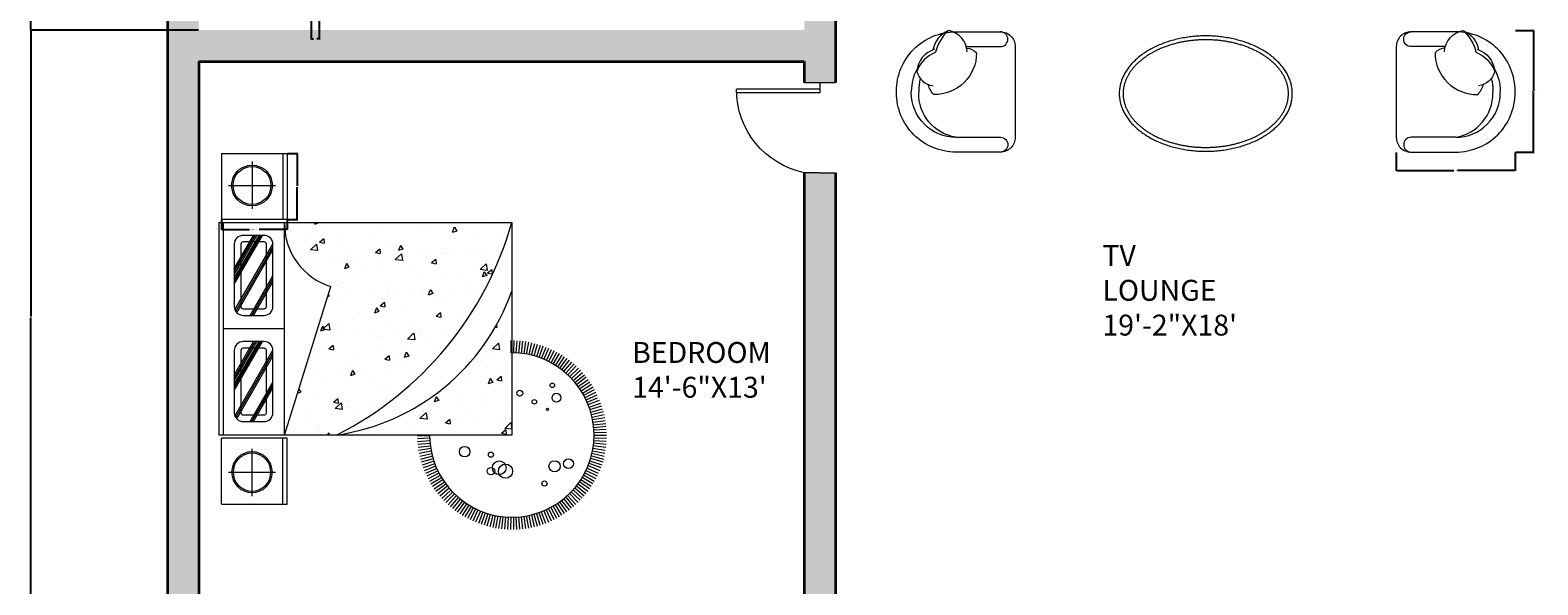
# Model space of a CAD drawing. Units: inches. Extents: x -9 to 646, y -802 to 47.
# Tile 14 of 17: x -9 to 424, y -412 to -253. Entities that reach past the tile are written whole.
import ezdxf

# ---------------------------------------------------------------- set-up
doc = ezdxf.new("R2010")
doc.units = ezdxf.units.IN
doc.header["$MEASUREMENT"] = 0
for name, color, linetype, lineweight in [('A-ANNO-DIMS', 2, 'Continuous', 18), ('A-AREA-IDEN', 7, 'Continuous', 18), ('A-DOOR', 4, 'Continuous', 18), ('A-FURN', 8, 'Continuous', 15), ('A-FURN-PATT', 252, 'Continuous', 9), ('A-WALL', 7, 'Continuous', 35), ('A-WALL-PATT', 5, 'Continuous', 9)]:
    doc.layers.add(name, color=color, linetype=linetype, lineweight=lineweight)
doc.styles.get("Standard").update_dxf_attribs({"font": 'arial.ttf'})
doc.dimstyles.get("Standard").update_dxf_attribs({"dimtxt": 0.18, "dimasz": 0.18, "dimexe": 0.18, "dimexo": 0.0625, "dimgap": 0.09, "dimtad": 0, "dimtih": 1, "dimtoh": 1, "dimdec": 0, "dimzin": 0, "dimdsep": 46, "dimlunit": 3, "dimtxsty": 'Standard', "dimcen": 0.09, "dimadec": 0, "dimazin": 0, "dimtfac": 1, "dimtdec": 0, "dimtofl": 0, "dimtmove": 0, "dimatfit": 3, "dimfxl": 1, "dimtolj": 1, "dimtzin": 0, "dimarcsym": 0})

# ---------------------------------------------------------------- blocks, each defined once
blk = doc.blocks.new('LOUNGE-ARMCHAIR')
for points in [[(13.85, 28.82, -0.356772), (19.23, 34.93, -0.249542), (23.66, 29.39, 9.61688)], [(19.23, 34.93, -0.14773), (22.9, 28.69, -0.213343), (28.28, 23.19, -0.178662)], [(14.08, 30.31), (4.27, 30.31, -0.414214), (2.13, 32.45), (2.13, 32.45, -0.414214), (4.27, 34.58)], [(13.98, 29.89, 0.165541), (11.16, 28.57, 0.425989), (23.39, 16.58, 0.121523), (25.07, 19.43, -7.115464)], [(23.19, 29.56, -0.306663), (28.28, 23.19, -0.30633), (23.63, 19.03, 0.872847)], [(28.19, 23.86, -0.130591), (29.88, 17.51), (29.88, 17.29)], [(27.29, 21.15, -0.072384), (27.75, 17.51), (27.75, 17.29)], [(17.07, 4.27, 0.372719), (27.75, 17.08), (27.75, 17.29)], [(17.07, 4.27, 0.414214), (29.88, 17.08), (29.88, 17.29)], [(17.07, 4.27), (4.27, 4.27, 0.414214), (2.13, 2.14), (2.13, 2.14, 0.414214), (4.27, 0)]]:
    blk.add_lwpolyline(points, format="xyb")
at = {"ltscale": 0.03}
blk.add_lwpolyline([(0, 17.29), (0, 4.27, 0.414214), (4.27, 0), (17.07, 0, 0.414214), (34.15, 17.08), (34.15, 17.29), (34.15, 17.51, 0.414214), (17.07, 34.58), (4.27, 34.58, 0.414214), (0, 30.31), (0, 17.29)], format="xyb", dxfattribs=at)
blk = doc.blocks.new('NIGHTSTAND-19')
for p, q in [((0, 18.94), (18.94, 18.94)), ((0, 18.94), (0, 0)), ((17.61, 18.94), (17.61, 0)), ((18.94, 18.94), (18.94, 0)), ((8.8, 16.66), (8.8, 3.04)), ((2.08, 9.77), (15.53, 9.77)), ((18.94, 0), (0, 0))]:
    blk.add_line(p, q)
for radius in [5.86, 5.44]:
    blk.add_circle((8.8, 9.77), radius)
blk = doc.blocks.new('DOOR-LEAF-24-WALL9')
for p, q in [((0, 0), (0, 24)), ((1, 0), (1, 24)), ((0, 0), (1, 0))]:
    blk.add_line(p, q)
blk.add_arc((0, -0.52), 24.52, 11.8123, 90)
blk = doc.blocks.new('*D18')
at = {"layer": 'A-ANNO-DIMS', "color": 0, "lineweight": -2, "transparency": 16777216}
for p, q in [((71.7, -249.89), (71.7, -255.77)), ((73.94, -249.89), (73.94, -255.77)), ((71.88, -255.59), (72.36, -255.59)), ((73.76, -255.59), (73.28, -255.59))]:
    blk.add_line(p, q, dxfattribs=at)
at = {"layer": 'A-ANNO-DIMS', "color": 0, "transparency": 16777216}
for points in [[(71.88, -255.56), (71.88, -255.62), (71.7, -255.59)], [(73.76, -255.56), (73.76, -255.62), (73.94, -255.59)]]:
    blk.add_solid(points, dxfattribs=at)
at = {"layer": 'Defpoints', "color": 0, "transparency": 16777216}
for p in [(71.7, -249.82), (73.94, -249.82), (73.94, -255.59)]:
    blk.add_point(p, dxfattribs=at)
at = {"layer": 'A-ANNO-DIMS', "color": 0, "transparency": 16777216, "insert": (72.82, -255.59), "char_height": 0.18, "attachment_point": 5}
blk.add_mtext('\\A1;2 TYP.', dxfattribs=at)
blk = doc.blocks.new('*D35')
at = {"layer": 'A-ANNO-DIMS', "color": 0, "lineweight": -2, "transparency": 16777216}
for p, q in [((417.7, -253.19), (423.06, -253.19)), ((422.88, -253.37), (422.88, -270.47)), ((422.88, -287.94), (422.88, -270.84)), ((417.7, -288.12), (423.06, -288.12))]:
    blk.add_line(p, q, dxfattribs=at)
at = {"layer": 'A-ANNO-DIMS', "color": 0, "transparency": 16777216}
for points in [[(422.85, -253.37), (422.91, -253.37), (422.88, -253.19)], [(422.85, -287.94), (422.91, -287.94), (422.88, -288.12)]]:
    blk.add_solid(points, dxfattribs=at)
at = {"layer": 'Defpoints', "color": 0, "transparency": 16777216}
for p in [(417.64, -253.19), (422.88, -253.19), (417.64, -288.12)]:
    blk.add_point(p, dxfattribs=at)
at = {"layer": 'A-ANNO-DIMS', "color": 0, "transparency": 16777216, "insert": (422.88, -270.65), "char_height": 0.18, "attachment_point": 5}
blk.add_mtext('\\A1;ARMCHAIR 35 TYP.', dxfattribs=at)
blk = doc.blocks.new('*D36')
at = {"layer": 'A-ANNO-DIMS', "color": 0, "lineweight": -2, "transparency": 16777216}
for p, q in [((383.49, -288.18), (383.49, -293.54)), ((417.64, -288.18), (417.64, -293.54)), ((383.67, -293.36), (400.04, -293.36)), ((417.46, -293.36), (401.09, -293.36))]:
    blk.add_line(p, q, dxfattribs=at)
at = {"layer": 'A-ANNO-DIMS', "color": 0, "transparency": 16777216}
for points in [[(383.67, -293.33), (383.67, -293.39), (383.49, -293.36)], [(417.46, -293.33), (417.46, -293.39), (417.64, -293.36)]]:
    blk.add_solid(points, dxfattribs=at)
at = {"layer": 'Defpoints', "color": 0, "transparency": 16777216}
for p in [(383.49, -288.12), (417.64, -288.12), (417.64, -293.36)]:
    blk.add_point(p, dxfattribs=at)
at = {"layer": 'A-ANNO-DIMS', "color": 0, "transparency": 16777216, "insert": (400.56, -293.36), "char_height": 0.18, "attachment_point": 5}
blk.add_mtext('\\A1;34 TYP.', dxfattribs=at)
blk = doc.blocks.new('*D41')
at = {"layer": 'A-ANNO-DIMS', "color": 0, "lineweight": -2, "transparency": 16777216}
for p, q in [((45.87, -307.54), (45.87, -310.49)), ((64.81, -307.54), (64.81, -310.49)), ((46.05, -310.31), (53.96, -310.31)), ((64.63, -310.31), (56.71, -310.31))]:
    blk.add_line(p, q, dxfattribs=at)
at = {"layer": 'A-ANNO-DIMS', "color": 0, "transparency": 16777216}
for points in [[(46.05, -310.28), (46.05, -310.34), (45.87, -310.31)], [(64.63, -310.28), (64.63, -310.34), (64.81, -310.31)]]:
    blk.add_solid(points, dxfattribs=at)
at = {"layer": 'Defpoints', "color": 0, "transparency": 16777216}
for p in [(45.87, -307.47), (64.81, -307.47), (64.81, -310.31)]:
    blk.add_point(p, dxfattribs=at)
at = {"layer": 'A-ANNO-DIMS', "color": 0, "transparency": 16777216, "insert": (55.34, -310.31), "char_height": 0.18, "attachment_point": 5}
blk.add_mtext('\\A1;NIGHTSTAND 19 TYP.', dxfattribs=at)
blk = doc.blocks.new('*D42')
at = {"layer": 'A-ANNO-DIMS', "color": 0, "lineweight": -2, "transparency": 16777216}
for p, q in [((64.87, -288.53), (67.83, -288.53)), ((67.65, -288.71), (67.65, -297.82)), ((67.65, -307.29), (67.65, -298.18)), ((64.87, -307.47), (67.83, -307.47))]:
    blk.add_line(p, q, dxfattribs=at)
at = {"layer": 'A-ANNO-DIMS', "color": 0, "transparency": 16777216}
for points in [[(67.62, -288.71), (67.68, -288.71), (67.65, -288.53)], [(67.62, -307.29), (67.68, -307.29), (67.65, -307.47)]]:
    blk.add_solid(points, dxfattribs=at)
at = {"layer": 'Defpoints', "color": 0, "transparency": 16777216}
for p in [(64.81, -288.53), (67.65, -288.53), (64.81, -307.47)]:
    blk.add_point(p, dxfattribs=at)
at = {"layer": 'A-ANNO-DIMS', "color": 0, "transparency": 16777216, "insert": (67.65, -298), "char_height": 0.18, "attachment_point": 5}
blk.add_mtext('\\A1;19 TYP.', dxfattribs=at)
blk = doc.blocks.new('*D54')
at = {"layer": 'A-ANNO-DIMS', "color": 0, "lineweight": -2, "transparency": 16777216}
for p, q in [((30.31, 7.93), (-9.06, 7.93)), ((-8.88, 7.75), (-8.88, -122.39)), ((-8.88, -252.89), (-8.88, -122.75)), ((39.31, -253.07), (-9.06, -253.07))]:
    blk.add_line(p, q, dxfattribs=at)
at = {"layer": 'A-ANNO-DIMS', "color": 0, "transparency": 16777216}
for points in [[(-8.91, 7.75), (-8.85, 7.75), (-8.88, 7.93)], [(-8.91, -252.89), (-8.85, -252.89), (-8.88, -253.07)]]:
    blk.add_solid(points, dxfattribs=at)
at = {"layer": 'Defpoints', "color": 0, "transparency": 16777216}
for p in [(30.37, 7.93), (-8.88, -253.07), (39.37, -253.07)]:
    blk.add_point(p, dxfattribs=at)
at = {"layer": 'A-ANNO-DIMS', "color": 0, "transparency": 16777216, "insert": (-8.88, -122.57), "char_height": 0.18, "attachment_point": 5}
blk.add_mtext('\\A1;261', dxfattribs=at)
blk = doc.blocks.new('*D55')
at = {"layer": 'A-ANNO-DIMS', "color": 0, "lineweight": -2, "transparency": 16777216}
for p, q in [((39.31, -253.07), (-9.06, -253.07)), ((-8.88, -253.25), (-8.88, -335.39)), ((-8.88, -417.89), (-8.88, -335.75)), ((39.31, -418.07), (-9.06, -418.07))]:
    blk.add_line(p, q, dxfattribs=at)
at = {"layer": 'A-ANNO-DIMS', "color": 0, "transparency": 16777216}
for points in [[(-8.91, -253.25), (-8.85, -253.25), (-8.88, -253.07)], [(-8.91, -417.89), (-8.85, -417.89), (-8.88, -418.07)]]:
    blk.add_solid(points, dxfattribs=at)
at = {"layer": 'Defpoints', "color": 0, "transparency": 16777216}
for p in [(39.37, -253.07), (-8.88, -418.07), (39.37, -418.07)]:
    blk.add_point(p, dxfattribs=at)
at = {"layer": 'A-ANNO-DIMS', "color": 0, "transparency": 16777216, "insert": (-8.88, -335.57), "char_height": 0.18, "attachment_point": 5}
blk.add_mtext('\\A1;165', dxfattribs=at)

msp = doc.modelspace()

# ---------------------------------------------------------------- hatches: boundary and pattern name
at = {"layer": 'A-FURN-PATT'}
h = msp.add_hatch(dxfattribs=at)
h.set_pattern_fill('AR-CONC', color=256, scale=0.084177, angle=270, style=0)
h.set_pattern_definition([(220, (4822.164, 410.692), (1.341702, -15.33573), [1.60357, -17.63926]), (275, (4822.164, 410.692), (-16.082546, 2.96663), [1.282855, -14.111407]), (169.549, (4822.275, 409.414), (-14.74077, -12.369157), [1.362823, -14.991055]), (223.8158, (4817.887, 410.692), (3.53899, -22.81858), [2.40535, -26.45889]), (173.3644, (4818.182, 408.79), (-20.8275, -19.98394), [2.04423, -22.48658]), (278.816, (4817.887, 410.692), (-20.82747, -19.98397), [1.92428, -21.16711]), (249, (4818.956, 408.554), (8.60839, -12.762463), [1.60357, -17.63926]), (304, (4818.956, 408.554), (-15.50436, -5.2023), [1.282855, -14.111407]), (198.5486, (4819.674, 407.49), (-6.89601, -17.964728), [1.362823, -14.991055]), (232.5, (4822.1636, 410.692), (-7.1175767, -0.259989), [0, -13.94036, 0, -14.325216, 0, -14.164859]), (262.5, (4822.1636, 410.692), (-8.432885, -5.624669), [0, -8.167511, 0, -13.619646, 0, -5.398682]), (302.5, (4822.1636, 415.46), (0.4822276, -11.413589), [0, -5.34523, 0, -16.677117, 0, -22.129252]), (312.5, (4822.164, 417.598), (-2.140322, -12.469048), [0, -6.948799, 0, -11.075316, 0, -15.714976])])
edge = h.paths.add_edge_path()
edge.add_ellipse((82.85, -308.76), major_axis=(-13.31, -13.31), ratio=1, start_angle=-43.8468, end_angle=28.0453, ccw=False)
edge.add_line((64.04, -309.14), (64.04, -308.38))
edge.add_line((64.04, -308.38), (129.32, -308.38))
edge.add_ellipse((34.64, -281.57), major_axis=(-69.58, -69.58), ratio=1, start_angle=71.7955, end_angle=119.1914, ccw=False)
edge.add_line((79, -369.41), (64.04, -369.41))
edge.add_line((64.04, -369.41), (77.36, -326.76))
edge = h.paths.add_edge_path()
edge.add_line((129.32, -328.06), (129.32, -369.41))
edge.add_line((129.32, -369.41), (79, -369.41))
edge.add_ellipse((69.95, -307.11), major_axis=(-44.51, 44.51), ratio=1, start_angle=143.2583, end_angle=205.5572)
h = msp.add_hatch(dxfattribs=at)
h.set_pattern_fill('ANSI31', color=256, scale=3.36678, angle=15.0416, style=0)
h.paths.add_polyline_path([(49.57, -324.21), (49.57, -326.3), (57.79, -312.05), (56.58, -312.05)])
h = msp.add_hatch(dxfattribs=at)
h.set_pattern_fill('ANSI31', color=256, scale=3.365103, angle=15.04163, style=0)
h.paths.add_polyline_path([(49.57, -321.48), (49.57, -323.57), (56.22, -312.05), (55.01, -312.05)])
h = msp.add_hatch(dxfattribs=at)
h.set_pattern_fill('ANSI31', color=256, scale=3.36781, angle=15.0416, style=0)
h.paths.add_polyline_path([(49.72, -333.35), (49.74, -333.38), (49.77, -333.46), (49.8, -333.53), (49.83, -333.61), (49.87, -333.68), (49.91, -333.75), (49.95, -333.82), (50, -333.89), (50.05, -333.96), (50.1, -334.03), (50.15, -334.09), (50.2, -334.16), (50.26, -334.22), (50.31, -334.28), (50.37, -334.33), (60.68, -316.43), (60.68, -314.57), (60.67, -314.4), (60.67, -314.36)])
h = msp.add_hatch(dxfattribs=at)
h.set_pattern_fill('ANSI31', color=256, scale=3.366878, angle=15.04163, style=0)
h.paths.add_polyline_path([(54.04, -335.02), (55.24, -335.02), (60.68, -325.59), (60.68, -323.5)])
h = msp.add_hatch(dxfattribs=at)
h.set_pattern_fill('ANSI31', color=256, scale=3.368112, angle=15.04163, style=0)
h.paths.add_polyline_path([(49.57, -354.72), (49.57, -356.81), (57.79, -342.56), (56.58, -342.56)])
h = msp.add_hatch(dxfattribs=at)
h.set_pattern_fill('ANSI31', color=256, scale=3.36656, angle=15.0416, style=0)
h.paths.add_polyline_path([(49.57, -351.99), (49.57, -354.08), (56.22, -342.56), (55.01, -342.56)])
h = msp.add_hatch(dxfattribs=at)
h.set_pattern_fill('ANSI31', color=256, scale=3.369047, angle=15.04163, style=0)
h.paths.add_polyline_path([(49.72, -363.86), (49.74, -363.9), (49.77, -363.97), (49.8, -364.05), (49.83, -364.12), (49.87, -364.2), (49.91, -364.27), (49.95, -364.34), (50, -364.41), (50.05, -364.48), (50.1, -364.54), (50.15, -364.61), (50.2, -364.67), (50.26, -364.73), (50.31, -364.79), (50.37, -364.84), (60.68, -346.95), (60.68, -345.09), (60.67, -344.91), (60.67, -344.87)])
h = msp.add_hatch(dxfattribs=at)
h.set_pattern_fill('ANSI31', color=256, scale=3.36815, angle=15.0416, style=0)
h.paths.add_polyline_path([(54.04, -365.53), (55.24, -365.53), (60.68, -356.1), (60.68, -354.01)])
at = {"layer": 'A-WALL-PATT'}
h = msp.add_hatch(color=256, dxfattribs=at)
h.dxf.hatch_style = 1
h.paths.add_polyline_path([(73.4, -418.07), (63.37, -418.07), (63.37, -487.07), (63.35, -496.07), (67.87, -496.07), (67.87, -427.07), (73.4, -427.07)])
h.paths.add_polyline_path([(73.87, -487.07), (67.87, -487.07), (67.87, -496.07), (73.87, -496.07)])
h.paths.add_polyline_path([(39.37, -496.07), (39.35, -496.07), (39.35, -487.07), (30.37, -487.07), (30.37, -646.07), (69.62, -646.07), (69.62, -637.07), (39.37, -637.07)])
h.paths.add_polyline_path([(158.27, -637.07), (105.62, -637.07), (105.62, -646.07), (158.27, -646.07)])
h.paths.add_polyline_path([(286.47, -637.07), (194.27, -637.07), (194.27, -646.07), (286.47, -646.07)])
h.paths.add_polyline_path([(357.37, -552.07), (352.87, -552.07), (348.37, -552.07), (348.37, -637.07), (322.47, -637.07), (322.47, -646.07), (357.37, -646.07)])
h.paths.add_polyline_path([(357.37, -459.07), (352.87, -459.07), (348.37, -459.07), (348.37, -526.07), (357.37, -526.07), (357.37, -520.07), (363.37, -520.07), (363.37, -511.07), (357.37, -511.07)], flags=17)
h.paths.add_polyline_path([(39.37, -262.07), (213.37, -262.07), (213.37, -268.07), (222.37, -268.07), (222.37, -247.07), (213.37, -247.07), (213.37, -253.07), (39.37, -253.07), (39.37, -1.07), (222.37, -1.07), (222.37, 7.93), (30.37, 7.93), (30.37, -427.07), (39.36, -427.07), (39.36, -418.07)])
h.paths.add_polyline_path([(570.37, -149.32), (561.37, -149.32), (561.37, -161.07), (433.37, -161.07), (433.37, -165.57), (433.37, -170.07), (438.37, -170.07), (438.37, -176.07), (447.37, -176.07), (447.37, -170.07), (561.37, -170.07), (561.37, -229.57), (570.37, -229.57)])
h.paths.add_polyline_path([(570.37, -289.57), (561.37, -289.57), (561.37, -349.07), (479.37, -349.07), (479.37, -353.57), (479.37, -358.07), (561.37, -358.07), (561.37, -418.07), (447.37, -418.07), (447.37, -358.07), (453.37, -358.07), (453.37, -349.07), (447.37, -349.07), (447.37, -202.07), (442.87, -202.07), (438.37, -202.07), (438.37, -427.07), (561.37, -427.07), (561.37, -451.07), (570.37, -451.07)])
h.paths.add_polyline_path([(570.37, -496.07), (570.37, -487.07), (561.37, -487.07), (561.37, -511.07), (411.37, -511.07), (411.37, -515.57), (411.37, -520.07), (570.37, -520.07)])
h = msp.add_hatch(color=256, dxfattribs=at)
h.dxf.hatch_style = 1
h.paths.add_polyline_path([(363.37, -418.07), (222.37, -418.07), (222.37, -294.07), (217.87, -294.07), (213.37, -294.07), (213.37, -418.07), (101.62, -418.07), (101.62, -427.07), (135.37, -427.07), (135.37, -487.07), (99.87, -487.07), (99.87, -491.57), (99.87, -496.07), (135.37, -496.07), (135.37, -568.07), (39.37, -568.07), (39.37, -496.07), (39.35, -496.07), (39.35, -487.07), (30.37, -487.07), (30.37, -646.07), (69.62, -646.07), (69.62, -637.07), (39.37, -637.07), (39.37, -577.07), (135.37, -577.07), (135.37, -605.07), (137.62, -605.07), (139.87, -605.07), (139.87, -427.07), (348.37, -427.07), (348.37, -433.07), (357.37, -433.07), (357.37, -427.07), (363.37, -427.07)])

# ---------------------------------------------------------------- linework, layer by layer
at = {"layer": 'A-DOOR'}
for p, q in [((213.37, -268.07), (222.37, -268.07)), ((217.87, -268.07), (217.87, -270.07)), ((217.87, -294.07), (213.37, -294.07)), ((217.87, -294.07), (222.37, -294.07))]:
    msp.add_line(p, q, dxfattribs=at)
at = {"layer": 'A-FURN'}
for p, q in [((45.14, -308.38), (45.14, -369.41)), ((45.14, -308.38), (129.32, -308.38)), ((46.52, -369.41), (46.52, -308.38)), ((64.04, -369.41), (64.04, -308.38)), ((129.32, -308.38), (129.32, -369.41)), ((64.04, -369.41), (77.36, -326.76)), ((64.04, -338.89), (46.52, -338.89)), ((129.11, -345.78), (129.11, -342.26)), ((129.86, -345.78), (129.97, -342.27)), ((130.6, -345.81), (130.83, -342.3)), ((131.35, -345.86), (131.68, -342.37)), ((132.09, -345.94), (132.54, -342.45)), ((132.83, -346.04), (133.39, -342.57)), ((133.57, -346.16), (134.23, -342.71)), ((134.3, -346.31), (135.08, -342.88)), ((135.03, -346.48), (135.91, -343.08)), ((135.75, -346.67), (136.74, -343.3)), ((136.47, -346.89), (137.56, -343.55)), ((137.18, -347.12), (138.38, -343.82)), ((137.88, -347.38), (139.18, -344.12)), ((138.57, -347.67), (139.98, -344.44)), ((139.26, -347.97), (140.76, -344.79)), ((139.93, -348.29), (141.53, -345.17)), ((140.59, -348.64), (142.29, -345.57)), ((141.24, -349.01), (143.04, -345.99)), ((141.88, -349.39), (143.78, -346.43)), ((142.51, -349.8), (144.49, -346.9)), ((143.12, -350.23), (145.2, -347.39)), ((143.72, -350.67), (145.89, -347.91)), ((144.31, -351.14), (146.56, -348.44)), ((144.88, -351.62), (147.21, -349)), ((145.43, -352.12), (147.85, -349.57)), ((145.97, -352.64), (148.47, -350.17)), ((146.49, -353.18), (149.07, -350.78)), ((147, -353.73), (149.65, -351.42)), ((147.48, -354.29), (150.2, -352.07)), ((147.95, -354.88), (150.74, -352.74)), ((148.4, -355.47), (151.26, -353.43)), ((148.83, -356.08), (151.75, -354.13)), ((149.24, -356.71), (152.22, -354.84)), ((149.64, -357.34), (152.67, -355.58)), ((150.01, -357.99), (153.1, -356.32)), ((150.36, -358.65), (153.5, -357.08)), ((150.69, -359.32), (153.88, -357.85)), ((151, -360), (153.95, -358.75)), ((151.28, -360.69), (154.57, -359.42)), ((151.55, -361.39), (154.88, -360.23)), ((151.79, -362.1), (155.16, -361.04)), ((152.01, -362.82), (155.41, -361.86)), ((152.21, -363.54), (155.64, -362.69)), ((152.38, -364.26), (155.84, -363.52)), ((152.53, -364.99), (156.02, -364.36)), ((152.66, -365.73), (156.17, -365.21)), ((152.76, -366.47), (156.3, -366.06)), ((152.85, -367.21), (156.39, -366.91)), ((152.9, -367.96), (156.46, -367.77)), ((129.32, -369.41), (45.14, -369.41)), ((105.68, -369.61), (102.17, -369.61)), ((105.7, -370.36), (102.19, -370.47)), ((105.74, -371.11), (102.24, -371.33)), ((105.81, -371.85), (102.31, -372.18)), ((152.75, -372.43), (156.32, -372.93)), ((152.84, -371.69), (156.41, -372.07)), ((152.9, -370.95), (156.47, -371.21)), ((152.93, -370.2), (156.51, -370.35)), ((152.94, -368.71), (156.51, -368.63)), ((152.95, -369.45), (156.52, -369.49)), ((105.9, -372.59), (102.41, -373.04)), ((106.01, -373.33), (102.54, -373.89)), ((106.15, -374.07), (102.7, -374.73)), ((106.31, -374.8), (102.88, -375.57)), ((106.49, -375.52), (103.09, -376.4)), ((106.69, -376.24), (103.32, -377.23)), ((151.76, -376.8), (155.2, -377.97)), ((151.98, -376.09), (155.45, -377.14)), ((152.18, -375.37), (155.68, -376.31)), ((152.36, -374.64), (155.88, -375.47)), ((152.52, -373.91), (156.05, -374.63)), ((152.65, -373.17), (156.2, -373.78)), ((106.92, -376.95), (103.58, -378.05)), ((107.17, -377.66), (103.87, -378.86)), ((107.44, -378.35), (104.18, -379.66)), ((107.74, -379.04), (104.51, -380.45)), ((108.05, -379.72), (104.88, -381.23)), ((108.39, -380.39), (105.26, -381.99)), ((108.75, -381.04), (105.67, -382.75)), ((149.96, -380.9), (153.02, -382.64)), ((150.32, -380.24), (153.43, -381.88)), ((150.65, -379.57), (153.81, -381.11)), ((150.96, -378.89), (154.17, -380.33)), ((151.25, -378.2), (154.62, -379.59)), ((151.52, -377.51), (154.92, -378.78)), ((109.12, -381.69), (106.1, -383.49)), ((109.52, -382.32), (106.56, -384.21)), ((109.94, -382.94), (107.04, -384.93)), ((110.38, -383.54), (107.54, -385.62)), ((110.83, -384.14), (108.07, -386.3)), ((111.31, -384.71), (108.61, -386.97)), ((111.8, -385.28), (109.18, -387.61)), ((146.94, -385.16), (149.54, -387.52)), ((147.43, -384.59), (150.1, -386.87)), ((147.9, -384.01), (150.64, -386.21)), ((148.35, -383.42), (151.16, -385.52)), ((148.78, -382.81), (151.66, -384.82)), ((149.2, -382.18), (152.14, -384.11)), ((149.59, -381.55), (152.59, -383.38)), ((112.31, -385.82), (109.76, -388.24)), ((112.84, -386.35), (110.37, -388.85)), ((113.38, -386.86), (110.99, -389.44)), ((113.94, -387.36), (111.63, -390.01)), ((114.52, -387.84), (112.29, -390.56)), ((115.11, -388.29), (112.97, -391.08)), ((115.71, -388.73), (113.67, -391.59)), ((116.33, -389.15), (114.37, -392.07)), ((116.96, -389.56), (115.1, -392.54)), ((141.17, -389.86), (142.9, -392.91)), ((141.81, -389.47), (143.64, -392.47)), ((142.43, -389.07), (144.36, -392.01)), ((143.05, -388.64), (145.07, -391.52)), ((143.65, -388.2), (145.76, -391.01)), ((144.24, -387.73), (146.43, -390.48)), ((144.81, -387.25), (147.09, -389.93)), ((145.37, -386.75), (147.73, -389.35)), ((145.91, -386.24), (148.35, -388.76)), ((146.43, -385.71), (148.95, -388.15)), ((117.61, -389.94), (115.84, -392.97)), ((118.26, -390.3), (116.59, -393.39)), ((118.93, -390.63), (117.35, -393.78)), ((119.6, -390.95), (118.13, -394.14)), ((120.29, -391.25), (118.92, -394.49)), ((120.98, -391.52), (119.72, -394.8)), ((121.69, -391.78), (120.52, -395.09)), ((122.4, -392.01), (121.34, -395.36)), ((123.12, -392.21), (122.17, -395.6)), ((123.84, -392.4), (123, -395.81)), ((124.57, -392.56), (123.83, -396)), ((125.3, -392.7), (124.68, -396.16)), ((126.04, -392.81), (125.53, -396.29)), ((126.79, -392.91), (126.38, -396.4)), ((127.53, -392.97), (127.23, -396.48)), ((128.28, -393.02), (128.09, -396.53)), ((129.02, -393.04), (128.95, -396.55)), ((129.77, -393.04), (129.81, -396.55)), ((130.52, -393.01), (130.66, -396.52)), ((131.26, -392.96), (131.52, -396.47)), ((132.01, -392.89), (132.38, -396.38)), ((132.75, -392.79), (133.23, -396.27)), ((133.48, -392.67), (134.08, -396.14)), ((134.22, -392.53), (134.92, -395.97)), ((134.95, -392.36), (135.75, -395.78)), ((135.67, -392.17), (136.59, -395.56)), ((136.39, -391.96), (137.41, -395.32)), ((137.1, -391.72), (138.22, -395.05)), ((137.8, -391.47), (139.03, -394.76)), ((138.49, -391.19), (139.83, -394.44)), ((139.18, -390.89), (140.61, -394.09)), ((139.85, -390.56), (141.39, -393.72)), ((140.51, -390.22), (142.15, -393.33))]:
    msp.add_line(p, q, dxfattribs=at)
for points in [[(49.57, -314.57), (49.57, -332.49, 0.414214), (52.1, -335.02), (58.15, -335.02, 0.414214), (60.68, -332.49), (60.68, -314.57, 0.414214), (58.15, -312.05), (52.1, -312.05, 0.414214)], [(51.47, -314.57), (51.47, -332.49, 0.414214), (52.1, -333.12), (58.15, -333.12, 0.414214), (58.79, -332.49), (58.79, -314.57, 0.414214), (58.15, -313.94), (52.1, -313.94, 0.414214)], [(49.57, -345.09), (49.57, -363.01, 0.414214), (52.1, -365.53), (58.15, -365.53, 0.414214), (60.68, -363.01), (60.68, -345.09, 0.414214), (58.15, -342.56), (52.1, -342.56, 0.414214)], [(51.47, -345.09), (51.47, -363.01, 0.414214), (52.1, -363.64), (58.15, -363.64, 0.414214), (58.79, -363.01), (58.79, -345.09, 0.414214), (58.15, -344.46), (52.1, -344.46, 0.414214)]]:
    msp.add_lwpolyline(points, format="xyb", close=True, dxfattribs=at)
at = {"layer": 'A-FURN', "ltscale": 0.03}
msp.add_polyline3d([(353.61, -271.3, 0), (353.6, -270.99, 0), (353.59, -270.67, 0), (353.56, -270.36, 0), (353.53, -270.05, 0), (353.49, -269.74, 0), (353.44, -269.42, 0), (353.39, -269.11, 0), (353.32, -268.8, 0), (353.25, -268.49, 0), (353.16, -268.18, 0), (353.07, -267.88, 0), (352.97, -267.57, 0), (352.86, -267.26, 0), (352.74, -266.96, 0), (352.61, -266.66, 0), (352.47, -266.36, 0), (352.33, -266.06, 0), (352.18, -265.76, 0), (352.02, -265.47, 0), (351.85, -265.18, 0), (351.67, -264.89, 0), (351.48, -264.6, 0), (351.29, -264.31, 0), (351.08, -264.03, 0), (350.87, -263.75, 0), (350.66, -263.47, 0), (350.43, -263.2, 0), (350.2, -262.92, 0), (349.95, -262.66, 0), (349.7, -262.39, 0), (349.45, -262.13, 0), (349.18, -261.87, 0), (348.91, -261.61, 0), (348.63, -261.36, 0), (348.35, -261.11, 0), (348.06, -260.86, 0), (347.76, -260.62, 0), (347.45, -260.38, 0), (347.14, -260.15, 0), (346.82, -259.92, 0), (346.49, -259.69, 0), (346.16, -259.47, 0), (345.82, -259.25, 0), (345.47, -259.04, 0), (345.12, -258.83, 0), (344.77, -258.63, 0), (344.4, -258.43, 0), (344.03, -258.23, 0), (343.66, -258.04, 0), (343.28, -257.86, 0), (342.9, -257.68, 0), (342.51, -257.5, 0), (342.11, -257.33, 0), (341.71, -257.16, 0), (341.31, -257, 0), (340.9, -256.85, 0), (340.49, -256.69, 0), (340.07, -256.55, 0), (339.65, -256.41, 0), (339.23, -256.27, 0), (338.8, -256.14, 0), (338.37, -256.02, 0), (337.93, -255.9, 0), (337.49, -255.79, 0), (337.05, -255.68, 0), (336.61, -255.58, 0), (336.16, -255.48, 0), (335.71, -255.39, 0), (335.26, -255.31, 0), (334.8, -255.23, 0), (334.34, -255.15, 0), (333.88, -255.09, 0), (333.42, -255.02, 0), (332.96, -254.97, 0), (332.5, -254.92, 0), (332.03, -254.87, 0), (331.56, -254.83, 0), (331.09, -254.8, 0), (330.63, -254.78, 0), (330.16, -254.75, 0), (329.69, -254.74, 0), (329.22, -254.73, 0), (328.75, -254.73, 0), (328.28, -254.73, 0), (327.81, -254.74, 0), (327.34, -254.75, 0), (326.87, -254.78, 0), (326.4, -254.8, 0), (325.93, -254.83, 0), (325.46, -254.87, 0), (325, -254.92, 0), (324.53, -254.97, 0), (324.07, -255.02, 0), (323.61, -255.09, 0), (323.15, -255.15, 0), (322.69, -255.23, 0), (322.24, -255.31, 0), (321.78, -255.39, 0), (321.33, -255.48, 0), (320.89, -255.58, 0), (320.44, -255.68, 0), (320, -255.79, 0), (319.56, -255.9, 0), (319.12, -256.02, 0), (318.69, -256.14, 0), (318.26, -256.27, 0), (317.84, -256.41, 0), (317.42, -256.55, 0), (317, -256.69, 0), (316.59, -256.85, 0), (316.18, -257, 0), (315.78, -257.16, 0), (315.38, -257.33, 0), (314.98, -257.5, 0), (314.59, -257.68, 0), (314.21, -257.86, 0), (313.83, -258.04, 0), (313.46, -258.23, 0), (313.09, -258.43, 0), (312.73, -258.63, 0), (312.37, -258.83, 0), (312.02, -259.04, 0), (311.67, -259.25, 0), (311.34, -259.47, 0), (311, -259.69, 0), (310.68, -259.92, 0), (310.36, -260.15, 0), (310.04, -260.38, 0), (309.74, -260.62, 0), (309.44, -260.86, 0), (309.14, -261.11, 0), (308.86, -261.36, 0), (308.58, -261.61, 0), (308.31, -261.87, 0), (308.04, -262.13, 0), (307.79, -262.39, 0), (307.54, -262.66, 0), (307.3, -262.92, 0), (307.06, -263.2, 0), (306.84, -263.47, 0), (306.62, -263.75, 0), (306.41, -264.03, 0), (306.21, -264.31, 0), (306.01, -264.6, 0), (305.82, -264.89, 0), (305.65, -265.18, 0), (305.48, -265.47, 0), (305.32, -265.76, 0), (305.16, -266.06, 0), (305.02, -266.36, 0), (304.88, -266.66, 0), (304.75, -266.96, 0), (304.64, -267.26, 0), (304.53, -267.57, 0), (304.42, -267.88, 0), (304.33, -268.18, 0), (304.25, -268.49, 0), (304.17, -268.8, 0), (304.1, -269.11, 0), (304.05, -269.42, 0), (304, -269.74, 0), (303.96, -270.05, 0), (303.93, -270.36, 0), (303.9, -270.67, 0), (303.89, -270.99, 0), (303.89, -271.3, 0), (303.89, -271.61, 0), (303.9, -271.93, 0), (303.93, -272.24, 0), (303.96, -272.55, 0), (304, -272.87, 0), (304.05, -273.18, 0), (304.1, -273.49, 0), (304.17, -273.8, 0), (304.25, -274.11, 0), (304.33, -274.42, 0), (304.42, -274.73, 0), (304.53, -275.03, 0), (304.64, -275.34, 0), (304.75, -275.64, 0), (304.88, -275.94, 0), (305.02, -276.24, 0), (305.16, -276.54, 0), (305.32, -276.84, 0), (305.48, -277.13, 0), (305.65, -277.43, 0), (305.82, -277.72, 0), (306.01, -278, 0), (306.21, -278.29, 0), (306.41, -278.57, 0), (306.62, -278.85, 0), (306.84, -279.13, 0), (307.06, -279.41, 0), (307.3, -279.68, 0), (307.54, -279.95, 0), (307.79, -280.21, 0), (308.04, -280.48, 0), (308.31, -280.74, 0), (308.58, -280.99, 0), (308.86, -281.24, 0), (309.14, -281.49, 0), (309.44, -281.74, 0), (309.74, -281.98, 0), (310.04, -282.22, 0), (310.36, -282.45, 0), (310.68, -282.68, 0), (311, -282.91, 0), (311.34, -283.13, 0), (311.67, -283.35, 0), (312.02, -283.56, 0), (312.37, -283.77, 0), (312.73, -283.97, 0), (313.09, -284.17, 0), (313.46, -284.37, 0), (313.83, -284.56, 0), (314.21, -284.75, 0), (314.59, -284.93, 0), (314.98, -285.1, 0), (315.38, -285.27, 0), (315.78, -285.44, 0), (316.18, -285.6, 0), (316.59, -285.76, 0), (317, -285.91, 0), (317.42, -286.05, 0), (317.84, -286.19, 0), (318.26, -286.33, 0), (318.69, -286.46, 0), (319.12, -286.58, 0), (319.56, -286.7, 0), (320, -286.81, 0), (320.44, -286.92, 0), (320.89, -287.02, 0), (321.33, -287.12, 0), (321.78, -287.21, 0), (322.24, -287.3, 0), (322.69, -287.37, 0), (323.15, -287.45, 0), (323.61, -287.52, 0), (324.07, -287.58, 0), (324.53, -287.63, 0), (325, -287.68, 0), (325.46, -287.73, 0), (325.93, -287.77, 0), (326.4, -287.8, 0), (326.87, -287.83, 0), (327.34, -287.85, 0), (327.81, -287.86, 0), (328.28, -287.87, 0), (328.75, -287.87, 0), (329.22, -287.87, 0), (329.69, -287.86, 0), (330.16, -287.85, 0), (330.63, -287.83, 0), (331.09, -287.8, 0), (331.56, -287.77, 0), (332.03, -287.73, 0), (332.5, -287.68, 0), (332.96, -287.63, 0), (333.42, -287.58, 0), (333.88, -287.52, 0), (334.34, -287.45, 0), (334.8, -287.37, 0), (335.26, -287.3, 0), (335.71, -287.21, 0), (336.16, -287.12, 0), (336.61, -287.02, 0), (337.05, -286.92, 0), (337.49, -286.81, 0), (337.93, -286.7, 0), (338.37, -286.58, 0), (338.8, -286.46, 0), (339.23, -286.33, 0), (339.65, -286.19, 0), (340.07, -286.05, 0), (340.49, -285.91, 0), (340.9, -285.76, 0), (341.31, -285.6, 0), (341.71, -285.44, 0), (342.11, -285.27, 0), (342.51, -285.1, 0), (342.9, -284.93, 0), (343.28, -284.75, 0), (343.66, -284.56, 0), (344.03, -284.37, 0), (344.4, -284.17, 0), (344.77, -283.97, 0), (345.12, -283.77, 0), (345.47, -283.56, 0), (345.82, -283.35, 0), (346.16, -283.13, 0), (346.49, -282.91, 0), (346.82, -282.68, 0), (347.14, -282.45, 0), (347.45, -282.22, 0), (347.76, -281.98, 0), (348.06, -281.74, 0), (348.35, -281.49, 0), (348.63, -281.24, 0), (348.91, -280.99, 0), (349.18, -280.74, 0), (349.45, -280.48, 0), (349.7, -280.21, 0), (349.95, -279.95, 0), (350.2, -279.68, 0), (350.43, -279.41, 0), (350.66, -279.13, 0), (350.87, -278.85, 0), (351.08, -278.57, 0), (351.29, -278.29, 0), (351.48, -278, 0), (351.67, -277.72, 0), (351.85, -277.43, 0), (352.02, -277.13, 0), (352.18, -276.84, 0), (352.33, -276.54, 0), (352.47, -276.24, 0), (352.61, -275.94, 0), (352.74, -275.64, 0), (352.86, -275.34, 0), (352.97, -275.03, 0), (353.07, -274.73, 0), (353.16, -274.42, 0), (353.25, -274.11, 0), (353.32, -273.8, 0), (353.39, -273.49, 0), (353.44, -273.18, 0), (353.49, -272.87, 0), (353.53, -272.55, 0), (353.56, -272.24, 0), (353.59, -271.93, 0), (353.6, -271.61, 0), (353.61, -271.3, 0)], dxfattribs=at)
at = {"layer": 'A-FURN'}
msp.add_polyline3d([(352.5, -271.3, 0), (352.5, -271.13, 0), (352.49, -270.96, 0), (352.49, -270.79, 0), (352.48, -270.62, 0), (352.46, -270.45, 0), (352.45, -270.27, 0), (352.43, -270.1, 0), (352.4, -269.92, 0), (352.38, -269.75, 0), (352.35, -269.57, 0), (352.32, -269.4, 0), (352.28, -269.22, 0), (352.24, -269.04, 0), (352.2, -268.87, 0), (352.15, -268.69, 0), (352.11, -268.51, 0), (352.05, -268.33, 0), (352, -268.15, 0), (351.94, -267.97, 0), (351.87, -267.79, 0), (351.81, -267.61, 0), (351.73, -267.43, 0), (351.66, -267.25, 0), (351.58, -267.07, 0), (351.5, -266.88, 0), (351.41, -266.7, 0), (351.32, -266.52, 0), (351.23, -266.34, 0), (351.13, -266.16, 0), (351.03, -265.98, 0), (350.93, -265.8, 0), (350.82, -265.62, 0), (350.71, -265.43, 0), (350.59, -265.25, 0), (350.47, -265.08, 0), (350.35, -264.9, 0), (350.22, -264.72, 0), (350.09, -264.54, 0), (349.95, -264.36, 0), (349.81, -264.19, 0), (349.67, -264.01, 0), (349.52, -263.83, 0), (349.37, -263.66, 0), (349.22, -263.49, 0), (349.06, -263.31, 0), (348.89, -263.14, 0), (348.73, -262.97, 0), (348.56, -262.8, 0), (348.38, -262.63, 0), (348.2, -262.47, 0), (348.02, -262.3, 0), (347.83, -262.14, 0), (347.64, -261.97, 0), (347.45, -261.81, 0), (347.25, -261.65, 0), (347.05, -261.49, 0), (346.85, -261.33, 0), (346.64, -261.18, 0), (346.43, -261.02, 0), (346.22, -260.87, 0), (346, -260.72, 0), (345.78, -260.57, 0), (345.56, -260.42, 0), (345.33, -260.27, 0), (345.11, -260.13, 0), (344.87, -259.99, 0), (344.64, -259.85, 0), (344.4, -259.71, 0), (344.16, -259.57, 0), (343.92, -259.44, 0), (343.68, -259.3, 0), (343.43, -259.17, 0), (343.18, -259.05, 0), (342.93, -258.92, 0), (342.67, -258.8, 0), (342.42, -258.68, 0), (342.16, -258.56, 0), (341.9, -258.44, 0), (341.63, -258.33, 0), (341.37, -258.22, 0), (341.1, -258.11, 0), (340.83, -258, 0), (340.56, -257.9, 0), (340.29, -257.8, 0), (340.02, -257.7, 0), (339.74, -257.6, 0), (339.47, -257.51, 0), (339.19, -257.42, 0), (338.92, -257.33, 0), (338.64, -257.25, 0), (338.36, -257.16, 0), (338.08, -257.08, 0), (337.8, -257.01, 0), (337.53, -256.93, 0), (337.25, -256.86, 0), (336.96, -256.79, 0), (336.68, -256.72, 0), (336.4, -256.66, 0), (336.12, -256.6, 0), (335.84, -256.54, 0), (335.56, -256.48, 0), (335.27, -256.43, 0), (334.99, -256.38, 0), (334.7, -256.33, 0), (334.42, -256.28, 0), (334.13, -256.23, 0), (333.85, -256.19, 0), (333.56, -256.15, 0), (333.28, -256.11, 0), (332.99, -256.08, 0), (332.7, -256.05, 0), (332.42, -256.02, 0), (332.13, -255.99, 0), (331.84, -255.96, 0), (331.56, -255.94, 0), (331.27, -255.92, 0), (330.98, -255.9, 0), (330.69, -255.88, 0), (330.4, -255.87, 0), (330.12, -255.86, 0), (329.83, -255.85, 0), (329.54, -255.84, 0), (329.25, -255.84, 0), (328.96, -255.83, 0), (328.67, -255.83, 0), (328.39, -255.83, 0), (328.1, -255.84, 0), (327.81, -255.84, 0), (327.52, -255.85, 0), (327.23, -255.86, 0), (326.94, -255.88, 0), (326.66, -255.89, 0), (326.37, -255.91, 0), (326.08, -255.93, 0), (325.79, -255.95, 0), (325.51, -255.98, 0), (325.22, -256, 0), (324.93, -256.03, 0), (324.64, -256.06, 0), (324.36, -256.1, 0), (324.07, -256.13, 0), (323.79, -256.17, 0), (323.5, -256.21, 0), (323.22, -256.26, 0), (322.93, -256.3, 0), (322.65, -256.35, 0), (322.36, -256.4, 0), (322.08, -256.45, 0), (321.8, -256.51, 0), (321.51, -256.57, 0), (321.23, -256.63, 0), (320.95, -256.69, 0), (320.67, -256.76, 0), (320.39, -256.83, 0), (320.11, -256.9, 0), (319.83, -256.97, 0), (319.55, -257.05, 0), (319.27, -257.12, 0), (318.99, -257.21, 0), (318.71, -257.29, 0), (318.44, -257.38, 0), (318.16, -257.46, 0), (317.89, -257.56, 0), (317.61, -257.65, 0), (317.34, -257.75, 0), (317.07, -257.85, 0), (316.79, -257.95, 0), (316.52, -258.05, 0), (316.26, -258.16, 0), (315.99, -258.27, 0), (315.73, -258.38, 0), (315.46, -258.5, 0), (315.2, -258.62, 0), (314.95, -258.74, 0), (314.69, -258.86, 0), (314.44, -258.98, 0), (314.19, -259.11, 0), (313.94, -259.24, 0), (313.69, -259.37, 0), (313.45, -259.5, 0), (313.21, -259.64, 0), (312.97, -259.78, 0), (312.73, -259.92, 0), (312.5, -260.06, 0), (312.27, -260.2, 0), (312.04, -260.35, 0), (311.82, -260.49, 0), (311.6, -260.64, 0), (311.38, -260.79, 0), (311.17, -260.95, 0), (310.95, -261.1, 0), (310.75, -261.26, 0), (310.54, -261.41, 0), (310.34, -261.57, 0), (310.14, -261.73, 0), (309.95, -261.89, 0), (309.75, -262.05, 0), (309.57, -262.22, 0), (309.38, -262.38, 0), (309.2, -262.55, 0), (309.02, -262.72, 0), (308.85, -262.89, 0), (308.68, -263.06, 0), (308.52, -263.23, 0), (308.36, -263.4, 0), (308.2, -263.57, 0), (308.04, -263.75, 0), (307.9, -263.92, 0), (307.75, -264.1, 0), (307.61, -264.27, 0), (307.47, -264.45, 0), (307.34, -264.63, 0), (307.21, -264.81, 0), (307.08, -264.99, 0), (306.96, -265.17, 0), (306.84, -265.34, 0), (306.73, -265.53, 0), (306.62, -265.71, 0), (306.51, -265.89, 0), (306.41, -266.07, 0), (306.31, -266.25, 0), (306.21, -266.43, 0), (306.12, -266.61, 0), (306.04, -266.79, 0), (305.95, -266.97, 0), (305.87, -267.16, 0), (305.79, -267.34, 0), (305.72, -267.52, 0), (305.65, -267.7, 0), (305.59, -267.88, 0), (305.53, -268.06, 0), (305.47, -268.24, 0), (305.41, -268.42, 0), (305.36, -268.6, 0), (305.31, -268.78, 0), (305.27, -268.95, 0), (305.23, -269.13, 0), (305.19, -269.31, 0), (305.16, -269.49, 0), (305.13, -269.66, 0), (305.1, -269.84, 0), (305.08, -270.01, 0), (305.05, -270.19, 0), (305.04, -270.36, 0), (305.02, -270.53, 0), (305.01, -270.7, 0), (305, -270.88, 0), (305, -271.05, 0), (304.99, -271.22, 0), (304.99, -271.39, 0), (305, -271.56, 0), (305, -271.73, 0), (305.01, -271.9, 0), (305.02, -272.07, 0), (305.04, -272.24, 0), (305.05, -272.42, 0), (305.08, -272.59, 0), (305.1, -272.76, 0), (305.13, -272.94, 0), (305.16, -273.12, 0), (305.19, -273.29, 0), (305.23, -273.47, 0), (305.27, -273.65, 0), (305.31, -273.83, 0), (305.36, -274, 0), (305.41, -274.18, 0), (305.47, -274.36, 0), (305.53, -274.54, 0), (305.59, -274.72, 0), (305.65, -274.9, 0), (305.72, -275.08, 0), (305.79, -275.26, 0), (305.87, -275.45, 0), (305.95, -275.63, 0), (306.04, -275.81, 0), (306.12, -275.99, 0), (306.21, -276.17, 0), (306.31, -276.35, 0), (306.41, -276.53, 0), (306.51, -276.72, 0), (306.62, -276.9, 0), (306.73, -277.08, 0), (306.84, -277.26, 0), (306.96, -277.44, 0), (307.08, -277.62, 0), (307.21, -277.79, 0), (307.34, -277.97, 0), (307.47, -278.15, 0), (307.61, -278.33, 0), (307.75, -278.5, 0), (307.9, -278.68, 0), (308.04, -278.85, 0), (308.2, -279.03, 0), (308.36, -279.2, 0), (308.52, -279.37, 0), (308.68, -279.54, 0), (308.85, -279.71, 0), (309.02, -279.88, 0), (309.2, -280.05, 0), (309.38, -280.22, 0), (309.57, -280.38, 0), (309.75, -280.55, 0), (309.95, -280.71, 0), (310.14, -280.87, 0), (310.34, -281.03, 0), (310.54, -281.19, 0), (310.75, -281.35, 0), (310.95, -281.5, 0), (311.17, -281.66, 0), (311.38, -281.81, 0), (311.6, -281.96, 0), (311.82, -282.11, 0), (312.04, -282.25, 0), (312.27, -282.4, 0), (312.5, -282.54, 0), (312.73, -282.68, 0), (312.97, -282.82, 0), (313.21, -282.96, 0), (313.45, -283.1, 0), (313.69, -283.23, 0), (313.94, -283.36, 0), (314.19, -283.49, 0), (314.44, -283.62, 0), (314.69, -283.74, 0), (314.95, -283.87, 0), (315.2, -283.99, 0), (315.46, -284.1, 0), (315.73, -284.22, 0), (315.99, -284.33, 0), (316.26, -284.44, 0), (316.52, -284.55, 0), (316.79, -284.65, 0), (317.07, -284.76, 0), (317.34, -284.85, 0), (317.61, -284.95, 0), (317.89, -285.05, 0), (318.16, -285.14, 0), (318.44, -285.23, 0), (318.71, -285.31, 0), (318.99, -285.4, 0), (319.27, -285.48, 0), (319.55, -285.56, 0), (319.83, -285.63, 0), (320.11, -285.71, 0), (320.39, -285.78, 0), (320.67, -285.84, 0), (320.95, -285.91, 0), (321.23, -285.97, 0), (321.51, -286.03, 0), (321.8, -286.09, 0), (322.08, -286.15, 0), (322.36, -286.2, 0), (322.65, -286.25, 0), (322.93, -286.3, 0), (323.22, -286.35, 0), (323.5, -286.39, 0), (323.79, -286.43, 0), (324.07, -286.47, 0), (324.36, -286.51, 0), (324.64, -286.54, 0), (324.93, -286.57, 0), (325.22, -286.6, 0), (325.51, -286.63, 0), (325.79, -286.65, 0), (326.08, -286.67, 0), (326.37, -286.69, 0), (326.66, -286.71, 0), (326.94, -286.73, 0), (327.23, -286.74, 0), (327.52, -286.75, 0), (327.81, -286.76, 0), (328.1, -286.76, 0), (328.39, -286.77, 0), (328.67, -286.77, 0), (328.96, -286.77, 0), (329.25, -286.77, 0), (329.54, -286.76, 0), (329.83, -286.75, 0), (330.12, -286.74, 0), (330.4, -286.73, 0), (330.69, -286.72, 0), (330.98, -286.7, 0), (331.27, -286.68, 0), (331.56, -286.66, 0), (331.84, -286.64, 0), (332.13, -286.61, 0), (332.42, -286.59, 0), (332.7, -286.55, 0), (332.99, -286.52, 0), (333.28, -286.49, 0), (333.56, -286.45, 0), (333.85, -286.41, 0), (334.13, -286.37, 0), (334.42, -286.32, 0), (334.7, -286.28, 0), (334.99, -286.23, 0), (335.27, -286.17, 0), (335.56, -286.12, 0), (335.84, -286.06, 0), (336.12, -286, 0), (336.4, -285.94, 0), (336.68, -285.88, 0), (336.96, -285.81, 0), (337.25, -285.74, 0), (337.53, -285.67, 0), (337.8, -285.59, 0), (338.08, -285.52, 0), (338.36, -285.44, 0), (338.64, -285.35, 0), (338.92, -285.27, 0), (339.19, -285.18, 0), (339.47, -285.09, 0), (339.74, -285, 0), (340.02, -284.9, 0), (340.29, -284.81, 0), (340.56, -284.7, 0), (340.83, -284.6, 0), (341.1, -284.49, 0), (341.37, -284.39, 0), (341.63, -284.27, 0), (341.9, -284.16, 0), (342.16, -284.04, 0), (342.42, -283.93, 0), (342.67, -283.8, 0), (342.93, -283.68, 0), (343.18, -283.56, 0), (343.43, -283.43, 0), (343.68, -283.3, 0), (343.92, -283.16, 0), (344.16, -283.03, 0), (344.4, -282.89, 0), (344.64, -282.76, 0), (344.87, -282.61, 0), (345.11, -282.47, 0), (345.33, -282.33, 0), (345.56, -282.18, 0), (345.78, -282.03, 0), (346, -281.88, 0), (346.22, -281.73, 0), (346.43, -281.58, 0), (346.64, -281.42, 0), (346.85, -281.27, 0), (347.05, -281.11, 0), (347.25, -280.95, 0), (347.45, -280.79, 0), (347.64, -280.63, 0), (347.83, -280.47, 0), (348.02, -280.3, 0), (348.2, -280.13, 0), (348.38, -279.97, 0), (348.56, -279.8, 0), (348.73, -279.63, 0), (348.89, -279.46, 0), (349.06, -279.29, 0), (349.22, -279.12, 0), (349.37, -278.94, 0), (349.52, -278.77, 0), (349.67, -278.59, 0), (349.81, -278.42, 0), (349.95, -278.24, 0), (350.09, -278.06, 0), (350.22, -277.88, 0), (350.35, -277.71, 0), (350.47, -277.53, 0), (350.59, -277.35, 0), (350.71, -277.17, 0), (350.82, -276.99, 0), (350.93, -276.81, 0), (351.03, -276.62, 0), (351.13, -276.44, 0), (351.23, -276.26, 0), (351.32, -276.08, 0), (351.41, -275.9, 0), (351.5, -275.72, 0), (351.58, -275.54, 0), (351.66, -275.35, 0), (351.73, -275.17, 0), (351.81, -274.99, 0), (351.87, -274.81, 0), (351.94, -274.63, 0), (352, -274.45, 0), (352.05, -274.27, 0), (352.11, -274.09, 0), (352.15, -273.91, 0), (352.2, -273.74, 0), (352.24, -273.56, 0), (352.28, -273.38, 0), (352.32, -273.2, 0), (352.35, -273.03, 0), (352.38, -272.85, 0), (352.4, -272.68, 0), (352.43, -272.5, 0), (352.45, -272.33, 0), (352.46, -272.16, 0), (352.48, -271.98, 0), (352.49, -271.81, 0), (352.49, -271.64, 0), (352.5, -271.47, 0), (352.5, -271.3, 0)], dxfattribs=at)
for centre, radius in [((140.98, -355.14), 0.641), ((131.62, -357.39), 0.868), ((135.81, -359.87), 0.641), ((142.16, -358.7), 1.28), ((139.57, -362.02), 0.31), ((115.78, -374.2), 1.51), ((123.33, -375.07), 0.744), ((125.72, -378.83), 1.97), ((141.62, -378.4), 1.61), ((145.61, -377.65), 1.41), ((123.33, -379.8), 1.07), ((127.52, -379.8), 2.05), ((138.71, -383.36), 0.744)]:
    msp.add_circle(centre, radius, dxfattribs=at)
for centre, radius, start, end in [((82.85, -308.76), 18.82, 178.8468, 253.0453), ((34.64, -281.57), 98.4, 296.7955, 344.1914), ((69.95, -307.11), 62.95, 278.2583, 340.5572), ((129.32, -369.41), 23.63, 180.4973, 90.4973)]:
    msp.add_arc(centre, radius, start, end, dxfattribs=at)
at = {"layer": 'A-WALL'}
for p, q in [((30.37, 7.93), (30.37, -646.07)), ((222.37, -247.07), (222.37, -268.07)), ((39.37, -262.07), (213.37, -262.07)), ((39.37, -262.07), (39.37, -487.07)), ((213.37, -262.07), (213.37, -268.07)), ((213.37, -294.07), (213.37, -418.07)), ((222.37, -294.07), (222.37, -418.07))]:
    msp.add_line(p, q, dxfattribs=at)

# ---------------------------------------------------------------- block references
at = {"layer": 'A-DOOR', "extrusion": (0, 0, -1), "zscale": -1, "rotation": 270.0000000000001}
msp.add_blockref('DOOR-LEAF-24-WALL9', (-217.87, -270.07), dxfattribs=at)
at = {"layer": 'A-FURN', "extrusion": (0, 0, -1), "zscale": -1}
msp.add_blockref('LOUNGE-ARMCHAIR', (-274, -288.12), dxfattribs=at)
at = {"layer": 'A-FURN'}
for name, p in [('LOUNGE-ARMCHAIR', (383.49, -288.12)), ('NIGHTSTAND-19', (45.87, -307.47))]:
    msp.add_blockref(name, p, dxfattribs=at)
at = {"layer": 'A-FURN', "extrusion": (0, 0, -1), "zscale": -1, "rotation": 180}
msp.add_blockref('NIGHTSTAND-19', (-45.87, -370.32), dxfattribs=at)

# ---------------------------------------------------------------- texts
at = {"layer": 'A-AREA-IDEN', "insert": (299.04, -314.82), "char_height": 6, "attachment_point": 1}
msp.add_mtext_dynamic_manual_height_columns('TV LOUNGE\\P19\'-2"X18\'', width=0.3939, gutter_width=1, heights=[0], dxfattribs=at)
at = {"layer": 'A-AREA-IDEN', "insert": (163.9, -342.69), "char_height": 6, "attachment_point": 1}
msp.add_mtext('BEDROOM\\P14\'-6"X13\'', dxfattribs=at)

# ---------------------------------------------------------------- dimensions: what is measured, and where the dimension line sits
at = {"layer": 'A-ANNO-DIMS'}
for base, p1, p2, picture, middle in [((-8.88, -253.07), (30.37, 7.93), (39.37, -253.07), '*D54', (-8.88, -122.57)), ((-8.88, -418.07), (39.37, -253.07), (39.37, -418.07), '*D55', (-8.88, -335.57))]:
    dim = msp.add_linear_dim(base=base, p1=p1, p2=p2, angle=90, dimstyle='Standard', override={"dimdec": 0, "dimlfac": 1, "dimrnd": 0, "dimzin": 0, "dimdsep": 46, "dimlunit": 2}, dxfattribs=at)
    dim.commit()
    dim.dimension.update_dxf_attribs({"geometry": picture, "text_midpoint": middle})
for base, p1, p2, text, picture, middle in [((73.94, -255.59), (71.7, -249.82), (73.94, -249.82), '<> TYP.', '*D18', (72.82, -255.59)), ((417.64, -293.36), (383.49, -288.12), (417.64, -288.12), '<> TYP.', '*D36', (400.56, -293.36)), ((64.81, -310.31), (45.87, -307.47), (64.81, -307.47), 'NIGHTSTAND <> TYP.', '*D41', (55.34, -310.31))]:
    dim = msp.add_linear_dim(base=base, p1=p1, p2=p2, text=text, dimstyle='Standard', override={"dimdec": 0, "dimlfac": 1, "dimrnd": 0, "dimzin": 0, "dimdsep": 46, "dimlunit": 2}, dxfattribs=at)
    dim.commit()
    dim.dimension.update_dxf_attribs({"geometry": picture, "text_midpoint": middle})
for base, p1, p2, text, picture, middle in [((422.88, -253.19), (417.64, -288.12), (417.64, -253.19), 'ARMCHAIR <> TYP.', '*D35', (422.88, -270.65)), ((67.65, -288.53), (64.81, -307.47), (64.81, -288.53), '<> TYP.', '*D42', (67.65, -298))]:
    dim = msp.add_linear_dim(base=base, p1=p1, p2=p2, angle=90, text=text, dimstyle='Standard', override={"dimdec": 0, "dimlfac": 1, "dimrnd": 0, "dimzin": 0, "dimdsep": 46, "dimlunit": 2}, dxfattribs=at)
    dim.commit()
    dim.dimension.update_dxf_attribs({"geometry": picture, "text_midpoint": middle})

doc.saveas('drawing.dxf')
